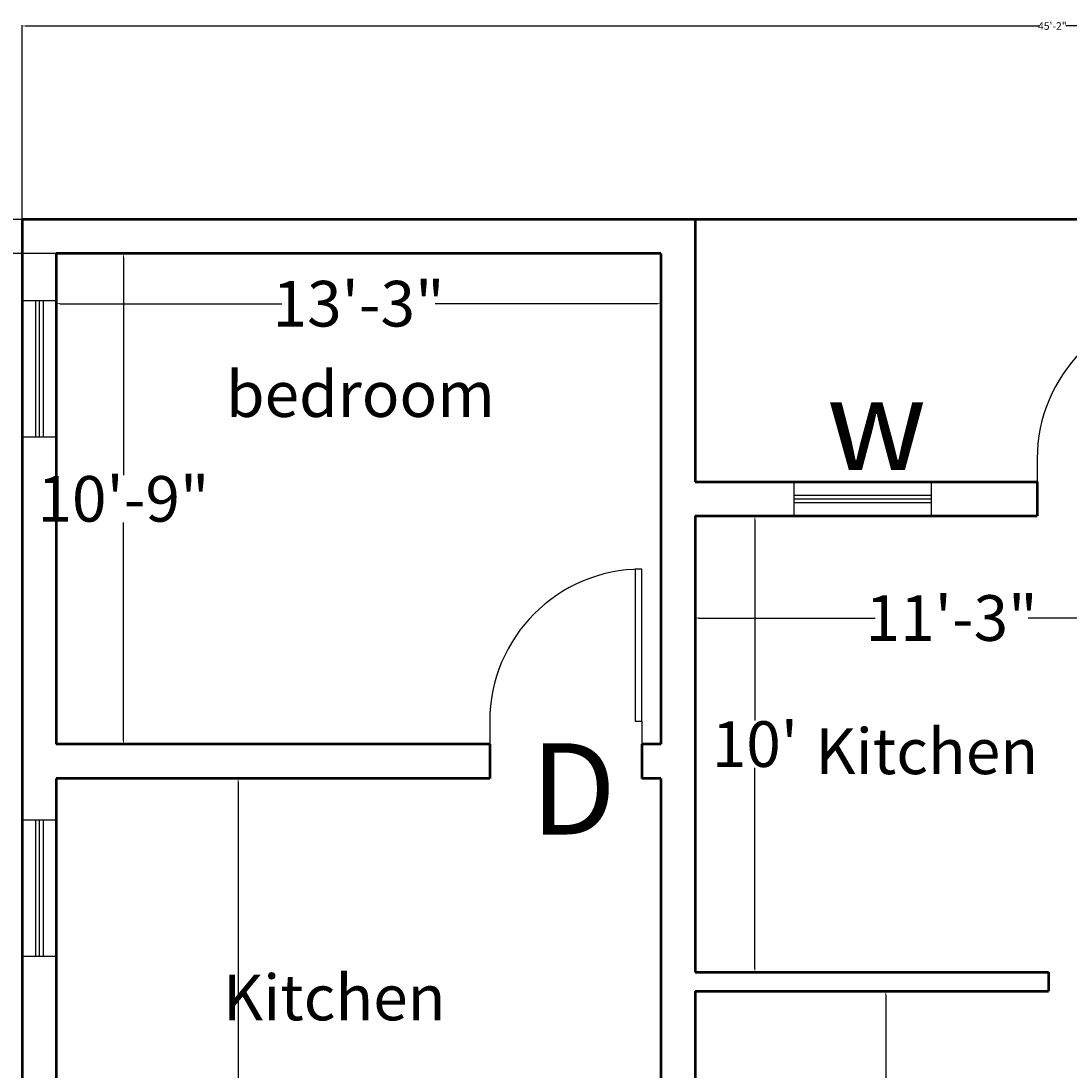
# Model space of a CAD drawing. Units: inches. Extents: x 409 to 7572, y 7 to 725.
# Tile 11 of 38: x 1696 to 1972, y 449 to 725. Entities that reach past the tile are written whole.
import ezdxf

# ---------------------------------------------------------------- set-up
doc = ezdxf.new("R2010")
doc.units = ezdxf.units.IN
doc.header["$MEASUREMENT"] = 0
for name, color, linetype, lineweight in [('A-ANNO-DIMS', 2, 'Continuous', 18), ('A-ANNO-SYMB', 3, 'Continuous', 25), ('A-AREA-IDEN', 7, 'Continuous', 25), ('A-DOOR', 3, 'Continuous', 25), ('A-GLAZ', 4, 'Continuous', 25), ('A-WALL', 7, 'Continuous', 50)]:
    doc.layers.add(name, color=color, linetype=linetype, lineweight=lineweight)
doc.styles.get("Standard").update_dxf_attribs({"font": 'arial.ttf'})
doc.dimstyles.get("Standard").update_dxf_attribs({"dimtxt": 2, "dimasz": 1, "dimexe": 0.18, "dimexo": 0.0625, "dimgap": 0.09, "dimtad": 0, "dimtih": 1, "dimtoh": 1, "dimdec": 0, "dimzin": 0, "dimdsep": 46, "dimlunit": 3, "dimtxsty": 'Standard', "dimcen": 0.09, "dimadec": 0, "dimazin": 0, "dimtfac": 1, "dimtdec": 0, "dimtofl": 0, "dimtmove": 0, "dimatfit": 3, "dimfxl": 1, "dimtolj": 1, "dimtzin": 0, "dimarcsym": 0})

# ---------------------------------------------------------------- blocks, each defined once
blk = doc.blocks.new('*U2')
for p, q in [((0, 0), (0, -6)), ((-40, 0), (-40, -6))]:
    blk.add_line(p, q)
blk.add_lwpolyline([(0, 0), (0, 40), (-1.75, 40), (-1.75, 0)], close=True)
blk.add_arc((0, 0), 40, 90, 180)
blk = doc.blocks.new('*D43')
at = {"layer": 'A-ANNO-DIMS', "color": 0, "lineweight": -2, "transparency": 16777216}
for p, q in [((1705.38, 663.53), (1723.15, 663.53)), ((1722.97, 662.53), (1722.97, 605.25)), ((1722.97, 535.53), (1722.97, 592.81)), ((1705.38, 534.53), (1723.15, 534.53))]:
    blk.add_line(p, q, dxfattribs=at)
at = {"layer": 'A-ANNO-DIMS', "color": 0, "transparency": 16777216}
for points in [[(1722.8, 662.53), (1723.14, 662.53), (1722.97, 663.53)], [(1722.8, 535.53), (1723.14, 535.53), (1722.97, 534.53)]]:
    blk.add_solid(points, dxfattribs=at)
at = {"layer": 'DEFPOINTS', "color": 0, "transparency": 16777216}
for p in [(1705.32, 663.53), (1705.32, 534.53), (1722.97, 534.53)]:
    blk.add_point(p, dxfattribs=at)
at = {"layer": 'A-ANNO-DIMS', "color": 0, "transparency": 16777216, "insert": (1722.97, 599.03), "char_height": 2, "attachment_point": 5}
blk.add_mtext('\\A1;{\\H6x;10\'-9"}', dxfattribs=at)
blk = doc.blocks.new('*D44')
at = {"layer": 'A-ANNO-DIMS', "color": 0, "lineweight": -2, "transparency": 16777216}
for p, q in [((1705.32, 663.47), (1705.32, 650.17)), ((1864.32, 663.47), (1864.32, 650.17)), ((1706.32, 650.35), (1764.68, 650.35)), ((1863.32, 650.35), (1804.96, 650.35))]:
    blk.add_line(p, q, dxfattribs=at)
at = {"layer": 'A-ANNO-DIMS', "color": 0, "transparency": 16777216}
for points in [[(1706.32, 650.52), (1706.32, 650.19), (1705.32, 650.35)], [(1863.32, 650.52), (1863.32, 650.19), (1864.32, 650.35)]]:
    blk.add_solid(points, dxfattribs=at)
at = {"layer": 'DEFPOINTS', "color": 0, "transparency": 16777216}
for p in [(1705.32, 663.53), (1864.32, 663.53), (1864.32, 650.35)]:
    blk.add_point(p, dxfattribs=at)
at = {"layer": 'A-ANNO-DIMS', "color": 0, "transparency": 16777216, "insert": (1784.82, 650.35), "char_height": 2, "attachment_point": 5}
blk.add_mtext('\\A1;{\\H6x;13\'-3"}', dxfattribs=at)
blk = doc.blocks.new('*D53')
at = {"layer": 'A-ANNO-DIMS', "color": 0, "lineweight": -2, "transparency": 16777216}
for p, q in [((1873.38, 594.53), (1889.26, 594.53)), ((1889.08, 593.53), (1889.08, 540.75)), ((1889.08, 475.53), (1889.08, 528.31)), ((1873.38, 474.53), (1889.26, 474.53))]:
    blk.add_line(p, q, dxfattribs=at)
at = {"layer": 'A-ANNO-DIMS', "color": 0, "transparency": 16777216}
for points in [[(1888.91, 593.53), (1889.24, 593.53), (1889.08, 594.53)], [(1888.91, 475.53), (1889.24, 475.53), (1889.08, 474.53)]]:
    blk.add_solid(points, dxfattribs=at)
at = {"layer": 'DEFPOINTS', "color": 0, "transparency": 16777216}
for p in [(1873.32, 594.53), (1873.32, 474.53), (1889.08, 474.53)]:
    blk.add_point(p, dxfattribs=at)
at = {"layer": 'A-ANNO-DIMS', "color": 0, "transparency": 16777216, "insert": (1889.08, 534.53), "char_height": 2, "attachment_point": 5}
blk.add_mtext("\\A1;{\\H6x;10'}", dxfattribs=at)
blk = doc.blocks.new('*D55')
at = {"layer": 'A-ANNO-DIMS', "color": 0, "lineweight": -2, "transparency": 16777216}
for p, q in [((1762.26, 525.53), (1752.98, 525.53)), ((1753.16, 524.53), (1753.16, 428.65)), ((1753.16, 320.53), (1753.16, 416.42)), ((1770.26, 319.53), (1752.98, 319.53))]:
    blk.add_line(p, q, dxfattribs=at)
at = {"layer": 'A-ANNO-DIMS', "color": 0, "transparency": 16777216}
for points in [[(1752.99, 524.53), (1753.32, 524.53), (1753.16, 525.53)], [(1752.99, 320.53), (1753.32, 320.53), (1753.16, 319.53)]]:
    blk.add_solid(points, dxfattribs=at)
at = {"layer": 'DEFPOINTS', "color": 0, "transparency": 16777216}
for p in [(1762.32, 525.53), (1753.16, 319.53), (1770.32, 319.53)]:
    blk.add_point(p, dxfattribs=at)
at = {"layer": 'A-ANNO-DIMS', "color": 0, "transparency": 16777216, "insert": (1753.16, 422.53), "char_height": 2, "attachment_point": 5}
blk.add_mtext('\\A1;{\\H6x;17\'-2"}', dxfattribs=at)
blk = doc.blocks.new('*D51')
at = {"layer": 'A-ANNO-DIMS', "color": 0, "lineweight": -2, "transparency": 16777216}
for p, q in [((1873.32, 563.4), (1873.32, 567.87)), ((1874.32, 567.69), (1920.68, 567.69)), ((2007.32, 567.69), (1960.96, 567.69)), ((2008.32, 563.4), (2008.32, 567.87))]:
    blk.add_line(p, q, dxfattribs=at)
at = {"layer": 'A-ANNO-DIMS', "color": 0, "transparency": 16777216}
for points in [[(1874.32, 567.86), (1874.32, 567.52), (1873.32, 567.69)], [(2007.32, 567.86), (2007.32, 567.52), (2008.32, 567.69)]]:
    blk.add_solid(points, dxfattribs=at)
at = {"layer": 'DEFPOINTS', "color": 0, "transparency": 16777216}
for p in [(2008.32, 567.69), (1873.32, 563.33), (2008.32, 563.33)]:
    blk.add_point(p, dxfattribs=at)
at = {"layer": 'A-ANNO-DIMS', "color": 0, "transparency": 16777216, "insert": (1940.82, 567.69), "char_height": 2, "attachment_point": 5}
blk.add_mtext('\\A1;{\\H6x;11\'-3"}', dxfattribs=at)
blk = doc.blocks.new('*D56')
at = {"layer": 'A-ANNO-DIMS', "color": 0, "lineweight": -2, "transparency": 16777216}
for p, q in [((1927.58, 469.53), (1923.34, 469.53)), ((1923.52, 468.53), (1923.52, 409.65)), ((1923.52, 338.53), (1923.52, 397.42)), ((1928.76, 337.53), (1923.34, 337.53))]:
    blk.add_line(p, q, dxfattribs=at)
at = {"layer": 'A-ANNO-DIMS', "color": 0, "transparency": 16777216}
for points in [[(1923.35, 468.53), (1923.68, 468.53), (1923.52, 469.53)], [(1923.35, 338.53), (1923.68, 338.53), (1923.52, 337.53)]]:
    blk.add_solid(points, dxfattribs=at)
at = {"layer": 'DEFPOINTS', "color": 0, "transparency": 16777216}
for p in [(1927.64, 469.53), (1923.52, 337.53), (1928.82, 337.53)]:
    blk.add_point(p, dxfattribs=at)
at = {"layer": 'A-ANNO-DIMS', "color": 0, "transparency": 16777216, "insert": (1923.52, 403.53), "char_height": 2, "attachment_point": 5}
blk.add_mtext("\\A1;{\\H6x;11'}", dxfattribs=at)
blk = doc.blocks.new('*D62')
at = {"layer": 'A-ANNO-DIMS', "color": 0, "lineweight": -2, "transparency": 16777216}
for p, q in [((1696.32, 672.59), (1696.32, 723.56)), ((2238.32, 672.59), (2238.32, 723.56)), ((1697.32, 723.38), (1963.75, 723.38)), ((2237.32, 723.38), (1970.88, 723.38))]:
    blk.add_line(p, q, dxfattribs=at)
at = {"layer": 'A-ANNO-DIMS', "color": 0, "transparency": 16777216}
for points in [[(1697.32, 723.55), (1697.32, 723.22), (1696.32, 723.38)], [(2237.32, 723.55), (2237.32, 723.22), (2238.32, 723.38)]]:
    blk.add_solid(points, dxfattribs=at)
at = {"layer": 'DEFPOINTS', "color": 0, "transparency": 16777216}
for p in [(1696.32, 723.38), (1696.32, 672.53), (2238.32, 672.53)]:
    blk.add_point(p, dxfattribs=at)
at = {"layer": 'A-ANNO-DIMS', "color": 0, "transparency": 16777216, "insert": (1967.32, 723.38), "char_height": 2, "attachment_point": 5}
blk.add_mtext('\\A1;45\'-2"', dxfattribs=at)
blk = doc.blocks.new('*D48')
at = {"layer": 'A-ANNO-DIMS', "color": 0, "lineweight": -2, "transparency": 16777216}
for p, q in [((1696.26, 672.53), (1585.36, 672.53)), ((1585.54, 671.53), (1585.54, 544.65)), ((1585.54, 405.53), (1585.54, 532.42)), ((1696.26, 404.53), (1585.36, 404.53))]:
    blk.add_line(p, q, dxfattribs=at)
at = {"layer": 'A-ANNO-DIMS', "color": 0, "transparency": 16777216}
for points in [[(1585.37, 671.53), (1585.71, 671.53), (1585.54, 672.53)], [(1585.37, 405.53), (1585.71, 405.53), (1585.54, 404.53)]]:
    blk.add_solid(points, dxfattribs=at)
at = {"layer": 'DEFPOINTS', "color": 0, "transparency": 16777216}
for p in [(1696.32, 672.53), (1585.54, 404.53), (1696.32, 404.53)]:
    blk.add_point(p, dxfattribs=at)
at = {"layer": 'A-ANNO-DIMS', "color": 0, "transparency": 16777216, "insert": (1585.54, 538.53), "char_height": 2, "attachment_point": 5}
blk.add_mtext('\\A1;{\\H6x;22\'-4"}', dxfattribs=at)
blk = doc.blocks.new('*D37')
at = {"layer": 'A-ANNO-DIMS', "color": 0, "lineweight": -2, "transparency": 16777216}
for p, q in [((1696.26, 672.53), (1531.9, 672.53)), ((1532.08, 671.53), (1532.08, 420.75)), ((1532.08, 157.53), (1532.08, 408.31)), ((1696.26, 156.53), (1531.9, 156.53))]:
    blk.add_line(p, q, dxfattribs=at)
at = {"layer": 'A-ANNO-DIMS', "color": 0, "transparency": 16777216}
for points in [[(1531.91, 671.53), (1532.25, 671.53), (1532.08, 672.53)], [(1531.91, 157.53), (1532.25, 157.53), (1532.08, 156.53)]]:
    blk.add_solid(points, dxfattribs=at)
at = {"layer": 'DEFPOINTS', "color": 0, "transparency": 16777216}
for p in [(1696.32, 672.53), (1532.08, 156.53), (1696.32, 156.53)]:
    blk.add_point(p, dxfattribs=at)
at = {"layer": 'A-ANNO-DIMS', "color": 0, "transparency": 16777216, "insert": (1532.08, 414.53), "char_height": 2, "attachment_point": 5}
blk.add_mtext("\\A1;{\\H6x;43'}", dxfattribs=at)
blk = doc.blocks.new('WIN-36')
for p, q in [((1699.82, 514.65), (1699.82, 478.65)), ((1700.82, 514.65), (1700.82, 478.65)), ((1701.82, 514.65), (1701.82, 478.65))]:
    blk.add_line(p, q)
blk.add_lwpolyline([(1705.32, 514.65), (1705.32, 478.65), (1696.32, 478.65), (1696.32, 514.65)], close=True)
blk = doc.blocks.new('*D178')
at = {"layer": 'A-ANNO-DIMS', "color": 0, "lineweight": -2, "transparency": 16777216}
for p, q in [((1696.26, 672.53), (1609.89, 672.53)), ((1610.07, 671.53), (1610.07, 669.14)), ((1610.07, 664.53), (1610.07, 666.92)), ((1705.26, 663.53), (1609.89, 663.53))]:
    blk.add_line(p, q, dxfattribs=at)
at = {"layer": 'A-ANNO-DIMS', "color": 0, "transparency": 16777216}
for points in [[(1609.9, 671.53), (1610.24, 671.53), (1610.07, 672.53)], [(1609.9, 664.53), (1610.24, 664.53), (1610.07, 663.53)]]:
    blk.add_solid(points, dxfattribs=at)
at = {"layer": 'DEFPOINTS', "color": 0, "transparency": 16777216}
for p in [(1696.32, 672.53), (1610.07, 663.53), (1705.32, 663.53)]:
    blk.add_point(p, dxfattribs=at)
at = {"layer": 'A-ANNO-DIMS', "color": 0, "transparency": 16777216, "insert": (1610.07, 668.03), "char_height": 2, "attachment_point": 5}
blk.add_mtext('\\A1;0\'-9"', dxfattribs=at)

msp = doc.modelspace()

# ---------------------------------------------------------------- linework, layer by layer
at = {"layer": 'A-WALL'}
for p, q in [((2238.32, 672.53), (1696.32, 672.53)), ((1696.32, 672.53), (1696.32, 404.53)), ((1873.32, 672.53), (1873.32, 603.53)), ((1864.32, 663.53), (1705.32, 663.53)), ((1705.32, 663.53), (1705.32, 534.53)), ((1864.32, 663.53), (1864.32, 534.53)), ((1864.32, 663.53), (1864.32, 534.53)), ((1873.32, 603.53), (1963.32, 603.53)), ((1963.32, 603.53), (1963.32, 594.53)), ((1873.32, 594.53), (1963.32, 594.53)), ((1873.32, 594.53), (1873.32, 474.53)), ((1819.32, 534.53), (1705.32, 534.53)), ((1819.32, 534.53), (1819.32, 525.53)), ((1864.32, 534.53), (1859.32, 534.53)), ((1859.32, 534.53), (1859.32, 525.53)), ((1819.32, 525.53), (1705.32, 525.53)), ((1705.32, 525.53), (1705.32, 404.53)), ((1864.32, 525.53), (1859.32, 525.53)), ((1864.32, 525.53), (1864.32, 319.53)), ((1873.32, 474.53), (1966.32, 474.53)), ((1966.32, 474.53), (1966.32, 469.53)), ((1873.32, 469.53), (1966.32, 469.53)), ((1873.32, 469.53), (1873.32, 337.53))]:
    msp.add_line(p, q, dxfattribs=at)

# ---------------------------------------------------------------- block references
at = {"layer": 'A-DOOR'}
for p in [(2003.32, 609.53), (1859.32, 540.53)]:
    msp.add_blockref('*U2', p, dxfattribs=at)
at = {"layer": 'A-GLAZ'}
for p in [(0, 136.58), (0, 0)]:
    msp.add_blockref('WIN-36', p, dxfattribs=at)
at = {"layer": 'A-GLAZ', "rotation": 89.99999999999844}
msp.add_blockref('WIN-36', (2414.06, -1101.79), dxfattribs=at)

# ---------------------------------------------------------------- texts
at = {"layer": 'A-ANNO-SYMB', "char_height": 24, "attachment_point": 1}
for s, width, insert in [('w', 18.2582, (1907.95, 630.65)), ('D', 19.1972, (1830.04, 534.75))]:
    msp.add_mtext_dynamic_manual_height_columns(s, width=width, gutter_width=1, heights=[0], dxfattribs=dict(at, insert=insert))
at = {"layer": 'A-AREA-IDEN', "char_height": 12, "attachment_point": 1}
for s, width, insert in [('bedroom', 40.9017, (1749.98, 632.57)), ('Kitchen ', 61.5504, (1905.01, 538.64)), ('Kitchen ', 61.5504, (1749.14, 473.89))]:
    msp.add_mtext_dynamic_manual_height_columns(s, width=width, gutter_width=1, heights=[0], dxfattribs=dict(at, insert=insert))

# ---------------------------------------------------------------- dimensions: what is measured, and where the dimension line sits
at = {"layer": 'A-ANNO-DIMS'}
dim = msp.add_linear_dim(base=(1696.32, 723.38), p1=(2238.32, 672.53), p2=(1696.32, 672.53), dimstyle='Standard', override={"dimclrd": 0, "dimclre": 0, "dimclrt": 0}, dxfattribs=at)
dim.commit()
dim.dimension.update_dxf_attribs({"geometry": '*D62', "text_midpoint": (1967.32, 723.38)})
for base, p1, p2, picture, middle in [((1532.08, 156.53), (1696.32, 672.53), (1696.32, 156.53), '*D37', (1532.08, 414.53)), ((1585.54, 404.53), (1696.32, 672.53), (1696.32, 404.53), '*D48', (1585.54, 538.53)), ((1722.97, 534.53), (1705.32, 663.53), (1705.32, 534.53), '*D43', (1722.97, 599.03)), ((1889.08, 474.53), (1873.32, 594.53), (1873.32, 474.53), '*D53', (1889.08, 534.53)), ((1923.52, 337.53), (1927.64, 469.53), (1928.82, 337.53), '*D56', (1923.52, 403.53))]:
    dim = msp.add_linear_dim(base=base, p1=p1, p2=p2, angle=90, text='{\\H6x;<>}', dimstyle='Standard', override={"dimclrd": 0, "dimclre": 0, "dimclrt": 0}, dxfattribs=at)
    dim.commit()
    dim.dimension.update_dxf_attribs({"geometry": picture, "text_midpoint": middle})
dim = msp.add_linear_dim(base=(1610.07, 663.53), p1=(1696.32, 672.53), p2=(1705.32, 663.53), angle=90, dimstyle='Standard', override={"dimdec": 1, "dimlfac": 1, "dimrnd": 0, "dimzin": 1, "dimdsep": 46, "dimlunit": 4, "dimfrac": 2}, dxfattribs=at)
dim.commit()
dim.dimension.update_dxf_attribs({"geometry": '*D178', "text_midpoint": (1610.07, 668.03)})
for base, p1, p2, picture, middle in [((1864.32, 650.35), (1705.32, 663.53), (1864.32, 663.53), '*D44', (1784.82, 650.35)), ((2008.32, 567.69), (1873.32, 563.33), (2008.32, 563.33), '*D51', (1940.82, 567.69))]:
    dim = msp.add_linear_dim(base=base, p1=p1, p2=p2, text='{\\H6x;<>}', dimstyle='Standard', override={"dimclrd": 0, "dimclre": 0, "dimclrt": 0}, dxfattribs=at)
    dim.commit()
    dim.dimension.update_dxf_attribs({"geometry": picture, "text_midpoint": middle})
dim = msp.add_linear_dim(base=(1753.16, 319.53), p1=(1762.32, 525.53), p2=(1770.32, 319.53), angle=90, text='{\\H6x;<>}', dimstyle='Standard', override={"dimclrd": 0, "dimclre": 0, "dimclrt": 0}, dxfattribs=at)
dim.commit()
dim.dimension.update_dxf_attribs({"geometry": '*D55', "text_midpoint": (1753.16, 422.53), "dimtype": 160})

doc.saveas('drawing.dxf')
